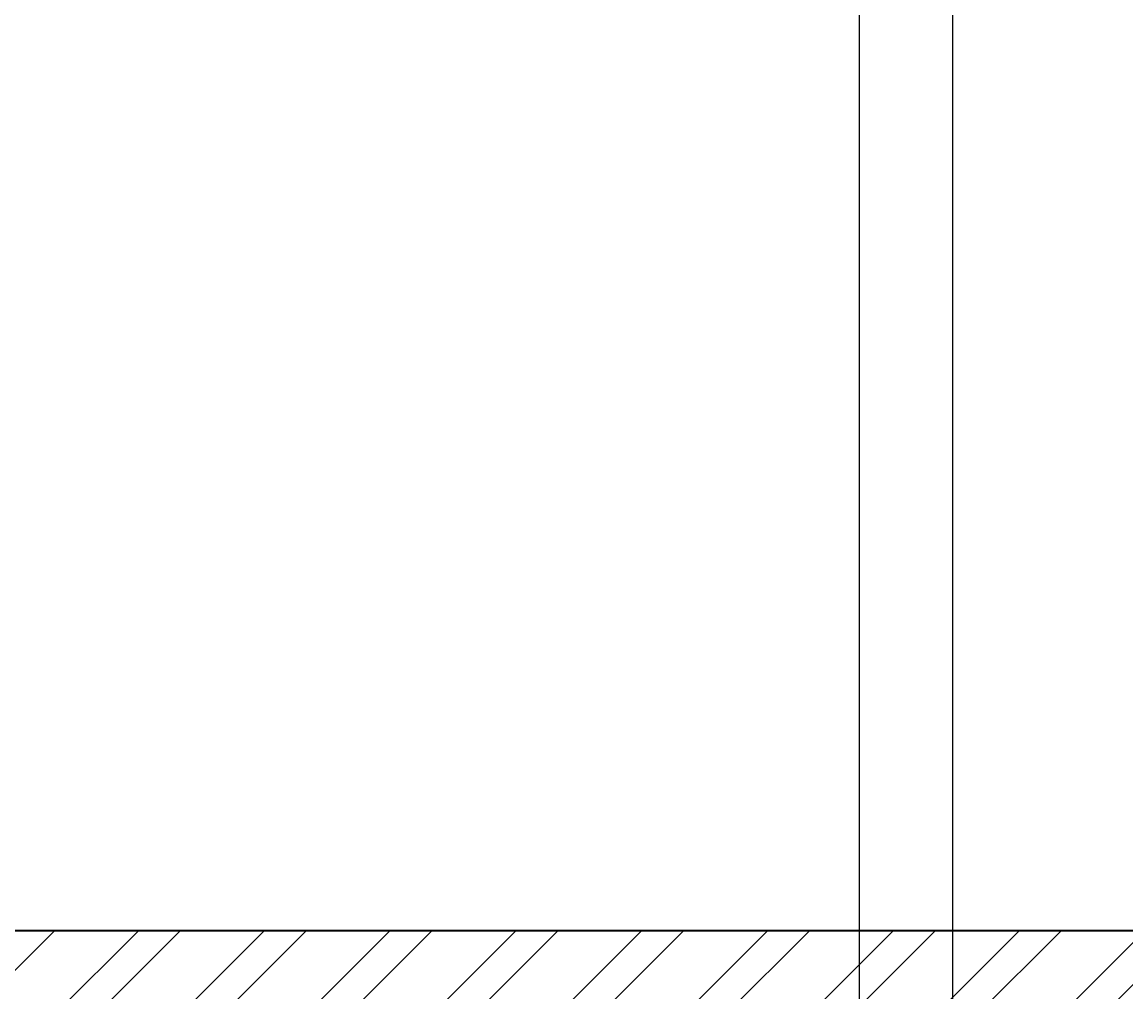
# Model space of a CAD drawing. Units: inches. Extents: x 2166 to 3588, y 1959 to 2628.
# Tile 8 of 13: x 3339 to 3457, y 2105 to 2209. Entities that reach past the tile are written whole.
import ezdxf

# ---------------------------------------------------------------- set-up
doc = ezdxf.new("R2010")
doc.units = ezdxf.units.IN
for name, color, linetype, lineweight in [('A-ANNO-DIMS', 2, 'Continuous', 18), ('A-WALL-PATT', 20, 'Continuous', 13), ('WALL', 40, 'Continuous', 35)]:
    doc.layers.add(name, color=color, linetype=linetype, lineweight=lineweight)
doc.styles.get("Standard").update_dxf_attribs({"font": 'arial.ttf'})
doc.dimstyles.get("Standard").update_dxf_attribs({"dimtxt": 0.18, "dimasz": 0.18, "dimexe": 0.18, "dimexo": 0.0625, "dimgap": 0.09, "dimtad": 0, "dimtih": 1, "dimtoh": 1, "dimdec": 4, "dimzin": 0, "dimdsep": 46, "dimtxsty": 'Standard', "dimcen": 0.09, "dimadec": 0, "dimazin": 0, "dimtfac": 1, "dimtdec": 4, "dimtofl": 0, "dimtmove": 0, "dimatfit": 3, "dimfxl": 1, "dimtolj": 1, "dimtzin": 0, "dimarcsym": 0})

# ---------------------------------------------------------------- blocks, each defined once
blk = doc.blocks.new('*D53')
at = {"layer": 'A-ANNO-DIMS', "color": 0, "lineweight": -2, "transparency": 16777216}
for p, q in [((3428.47, 2066.04), (3428.47, 2454.91)), ((3428.65, 2454.73), (3433.26, 2454.73)), ((3438.29, 2454.73), (3433.68, 2454.73)), ((3438.47, 2066.04), (3438.47, 2454.91))]:
    blk.add_line(p, q, dxfattribs=at)
at = {"layer": 'A-ANNO-DIMS', "color": 0, "transparency": 16777216}
for points in [[(3428.65, 2454.76), (3428.65, 2454.7), (3428.47, 2454.73)], [(3438.29, 2454.76), (3438.29, 2454.7), (3438.47, 2454.73)]]:
    blk.add_solid(points, dxfattribs=at)
at = {"layer": 'Defpoints', "color": 0, "transparency": 16777216}
for p in [(3438.47, 2454.73), (3428.47, 2065.98), (3438.47, 2065.98)]:
    blk.add_point(p, dxfattribs=at)
at = {"layer": 'A-ANNO-DIMS', "color": 0, "transparency": 16777216, "insert": (3433.47, 2454.73), "char_height": 0.18, "attachment_point": 5}
blk.add_mtext('\\A1;10', dxfattribs=at)

msp = doc.modelspace()

# ---------------------------------------------------------------- hatches: boundary and pattern name
at = {"layer": 'A-WALL-PATT'}
h = msp.add_hatch(dxfattribs=at)
h.set_pattern_fill('ANSI32', color=256)
h.paths.add_polyline_path([(3563.471, 2429.979), (3227.471, 2429.979), (3227.471, 2021.979), (3563.471, 2021.979)])
h.paths.add_polyline_path([(3236.471, 2420.979), (3554.471, 2420.979), (3554.471, 2111.979), (3236.471, 2111.979)], flags=16)
h.paths.add_polyline_path([(3236.471, 2102.979), (3554.471, 2102.979), (3554.471, 2030.979), (3236.471, 2030.979)], flags=16)
h.paths.add_polyline_path([(3518.471, 2085.283), (3518.471, 2067.979), (3458.471, 2067.979), (3458.471, 2085.283)], flags=0)
h.paths.add_polyline_path([(3434.656, 2082.283), (3442.194, 2082.283), (3442.194, 2087.514), (3434.656, 2087.514)], flags=8)
h.paths.add_polyline_path([(3522.671, 2094.512), (3521.752, 2052.984), (3545.541, 2052.457), (3546.46, 2093.986)], flags=8)

# ---------------------------------------------------------------- linework, layer by layer
at = {"layer": 'WALL'}
msp.add_line((3554.471, 2111.979), (3236.471, 2111.979), dxfattribs=at)

# ---------------------------------------------------------------- dimensions: what is measured, and where the dimension line sits
at = {"layer": 'A-ANNO-DIMS'}
dim = msp.add_linear_dim(base=(3438.471, 2454.729), p1=(3428.471, 2065.979), p2=(3438.471, 2065.979), dimstyle='Standard', override={"dimdec": 0, "dimlfac": 1, "dimrnd": 0, "dimzin": 0, "dimdsep": 46, "dimlunit": 2}, dxfattribs=at)
dim.commit()
dim.dimension.update_dxf_attribs({"geometry": '*D53', "text_midpoint": (3433.471, 2454.729)})

doc.saveas('drawing.dxf')
